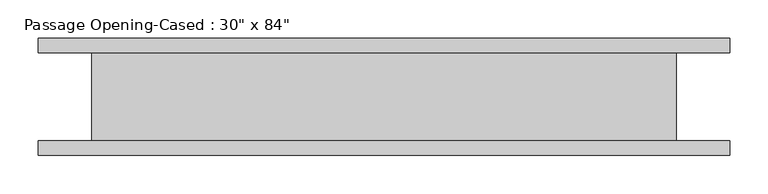
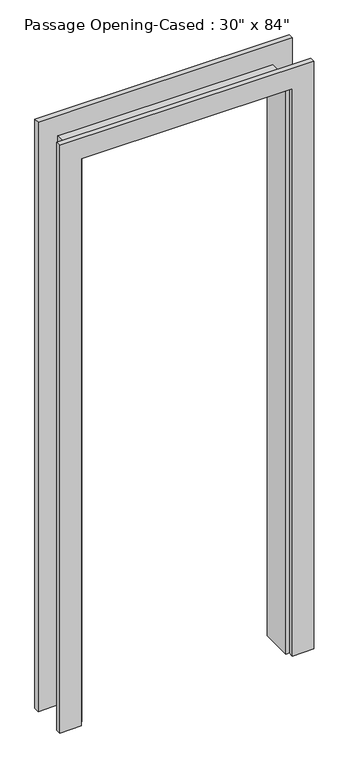
"""IFC4 building model written with IfcOpenShell, lengths in millimetres: proxy geometry."""

from ifc_helpers import new_model, si_unit, frame, origin, place, context, project, spatial, polyline, outline, extrude, faceted_brep, source, transform, mapped, element, save


def proxy_7d9a186d(model_context):
    return source(origin(), model_context, "Body", "SolidModel", [
        faceted_brep([(353.7613433, 57.15, 0.0), (372.8113433, 57.15, 0.0), (372.8113433, -57.15, 0.0), (353.7613433, -57.15, 0.0), (353.7613433, 57.15, 2114.55), (372.8113433, 57.15, 2133.6), (372.8113433, -57.15, 2133.6), (353.7613433, -57.15, 2114.55), (-370.1386567, 57.15, 2114.55), (-389.1886567, 57.15, 2133.6), (-389.1886567, -57.15, 2133.6), (-370.1386567, -57.15, 2114.55), (-370.1386567, 57.15, 0.0), (-370.1386567, -57.15, 0.0), (-389.1886567, -57.15, 0.0), (-389.1886567, 57.15, 0.0)], [[[0, 1, 2, 3]], [[1, 0, 4, 5]], [[2, 1, 5, 6]], [[3, 2, 6, 7]], [[0, 3, 7, 4]], [[5, 4, 8, 9]], [[6, 5, 9, 10]], [[7, 6, 10, 11]], [[4, 7, 11, 8]], [[12, 13, 14, 15]], [[9, 8, 12, 15]], [[10, 9, 15, 14]], [[11, 10, 14, 13]], [[8, 11, 13, 12]]]),
        extrude(outline(polyline([(0.0, 442.6613433), (2209.8, 442.6613433), (2209.8, -459.0386567), (0.0, -459.0386567), (0.0, -382.8386567), (2127.25, -382.8386567), (2127.25, 366.4613433), (0.0, 366.4613433), (0.0, 442.6613433)])), frame((0.0, 57.15, 0.0), z_axis=(0.0, 1.0, 0.0), x_axis=(0.0, 0.0, 1.0)), (0.0, 0.0, 1.0), 19.05),
        extrude(outline(polyline([(0.0, -382.8386567), (2127.25, -382.8386567), (2127.25, 366.4613433), (0.0, 366.4613433), (0.0, 442.6613433), (2203.45, 442.6613433), (2203.45, -459.0386567), (0.0, -459.0386567), (0.0, -382.8386567)])), frame((0.0, -76.2, 0.0), z_axis=(0.0, 1.0, 0.0), x_axis=(0.0, 0.0, 1.0)), (0.0, 0.0, 1.0), 19.05),
    ])


if __name__ == "__main__":
    model = new_model("IFC4")
    model_context = context("Model", 3, world=origin())
    ifc_project = project(units=[si_unit("LENGTHUNIT", "METRE", prefix="MILLI")], contexts=[model_context])
    site = spatial("IfcSite", under=ifc_project)
    building = spatial("IfcBuilding", under=site)
    placement = place(None, origin())
    proxy_shape = proxy_7d9a186d(model_context)
    element("IfcBuildingElementProxy", 1, Name="Passage Opening-Cased : 30\" x 84\"", ObjectType="Passage Opening-Cased : 30\" x 84\"", at=placement, inside=building, context=model_context, shape_type="MappedRepresentation", body=[
        mapped(proxy_shape, transform((0.0, 0.0, 0.0), x_axis=(1.0, 0.0, 0.0), y_axis=(0.0, 1.0, 0.0), z_axis=(0.0, 0.0, 1.0))),
    ])
    save(model, "model.ifc")

# Revit data of these elements
# Type "Passage Opening-Cased : 30\" x 84\""
#   Height = 7' - 0"
#   Trim Thickness = 0' - 0 3/4"
#   Trim Width = 0' - 3"
#   Width = 2' - 6"
#   Frame Material = Door - Frame
#   Default Elevation = 0
# Element 1 (IfcBuildingElementProxy, "Passage Opening-Cased : 30\" x 84\"")
#   Materials on its faces: "Door - Frame"
# Materials
#   "Door - Frame": colour RGB 118 70 51, transparency 0, Cost = 0
